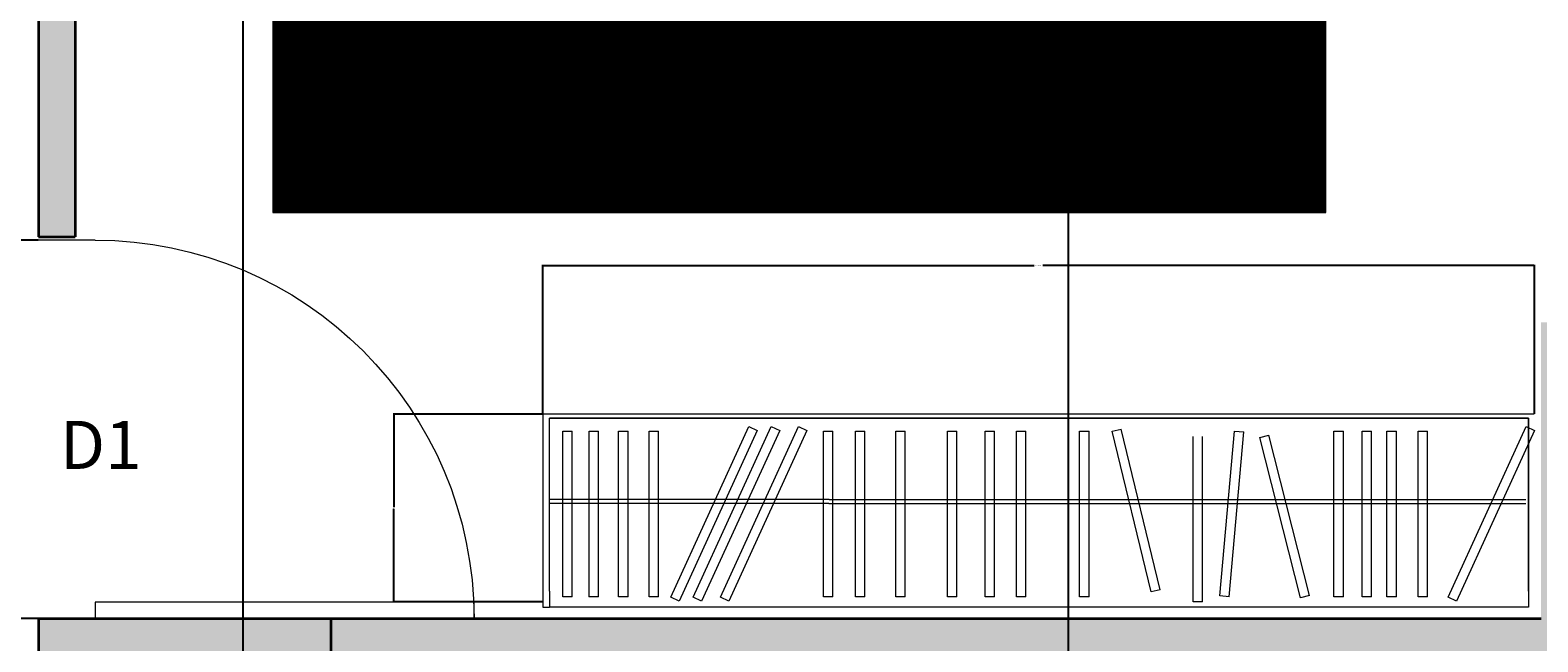
# Model space of a CAD drawing. Units: inches. Extents: x 192 to 1361, y -1362 to 367.
# Tile 20 of 23: x 783 to 1153, y -454 to -304. Entities that reach past the tile are written whole.
import ezdxf

# ---------------------------------------------------------------- set-up
doc = ezdxf.new("R2010")
doc.units = ezdxf.units.IN
doc.header["$MEASUREMENT"] = 0
for name, color, linetype, lineweight in [('A-ANNO-DIMS', 2, 'Continuous', 18), ('A-DOOR', 4, 'Continuous', 18), ('A-FLOR', 8, 'Continuous', 18), ('A-WALL-PATT', 250, 'Continuous', 13), ('closet', 32, 'Continuous', 18), ('text', 7, 'Continuous', 18), ('walls', 7, 'Continuous', 35)]:
    doc.layers.add(name, color=color, linetype=linetype, lineweight=lineweight)
doc.layers.add('A-FLOR-PATT', color=254, linetype='Continuous', lineweight=13, true_color=0xfeeab9)
doc.styles.get("Standard").update_dxf_attribs({"font": 'arial.ttf'})
doc.dimstyles.get("Standard").update_dxf_attribs({"dimtxt": 0.18, "dimasz": 0.18, "dimexe": 0.18, "dimexo": 0.0625, "dimgap": 0.09, "dimtad": 0, "dimtih": 1, "dimtoh": 1, "dimzin": 0, "dimdsep": 46, "dimlunit": 3, "dimtxsty": 'Standard', "dimcen": 0.09, "dimadec": 0, "dimazin": 0, "dimtfac": 1, "dimtofl": 0, "dimtmove": 0, "dimatfit": 3, "dimfxl": 1, "dimtolj": 1, "dimtzin": 0, "dimarcsym": 0})

# ---------------------------------------------------------------- blocks, each defined once
blk = doc.blocks.new('*U2')
for p, q in [((0, 0), (0, -6)), ((40, 0), (40, -6))]:
    blk.add_line(p, q)
blk.add_lwpolyline([(0, 0), (0, 40), (1.75, 40), (1.75, 0)], close=True)
blk.add_arc((0, 0), 40, 0, 90)
blk = doc.blocks.new('closet')
at = {"layer": 'closet'}
for p, q in [((-0.71, -5.58), (5.59, 8.19)), ((-0.23, 7.39), (-0.23, -6.57)), ((6.27, 7.88), (-0.04, -5.89)), ((5.59, 8.19), (6.27, 7.88)), ((7.92, 7.84), (8.68, 7.84)), ((7.92, 7.84), (7.92, -5.51)), ((8.68, 7.84), (8.68, -5.51)), ((10.44, 7.84), (11.2, 7.84)), ((10.44, 7.84), (10.44, -5.51)), ((11.2, 7.84), (11.2, -5.51)), ((12.45, 7.84), (13.21, 7.84)), ((12.45, 7.84), (12.45, -5.51)), ((13.21, 7.84), (13.21, -5.51)), ((14.71, 7.84), (15.47, 7.84)), ((14.71, 7.84), (14.71, -5.51)), ((15.47, 7.84), (15.47, -5.51)), ((17.44, 7.75), (18.17, 7.93)), ((17.44, 7.75), (20.73, -5.2)), ((18.17, 7.93), (21.46, -5.01)), ((23.92, 7.84), (22.75, -5.46)), ((24.67, 7.78), (23.51, -5.53)), ((23.92, 7.84), (24.67, 7.78)), ((26.09, 8.25), (26.09, -5.1)), ((26.84, 8.25), (26.84, -5.1)), ((30.22, 7.46), (33.37, -5.51)), ((35.23, 7.84), (35.23, -5.51)), ((35.99, 7.84), (35.99, -5.51)), ((40.33, 7.84), (40.33, -5.51)), ((41.08, 7.84), (41.08, -5.51)), ((42.85, 7.84), (42.85, -5.51)), ((43.61, 7.84), (43.61, -5.51)), ((45.9, 7.84), (45.9, -5.51)), ((46.65, 7.84), (46.65, -5.51)), ((50.07, 7.84), (50.07, -5.51)), ((50.82, 7.84), (50.82, -5.51)), ((53.32, 7.84), (53.32, -5.51)), ((54.08, 7.84), (54.08, -5.51)), ((55.9, 7.84), (55.9, -5.51)), ((56.65, 7.84), (56.65, -5.51)), ((57.99, -5.58), (64.3, 8.19)), ((64.97, 7.88), (58.67, -5.89)), ((60.19, -5.58), (66.49, 8.19)), ((67.17, 7.88), (60.87, -5.89)), ((62, -5.58), (68.3, 8.19)), ((68.98, 7.88), (62.67, -5.89)), ((69.96, 7.84), (69.96, -5.51)), ((70.72, 7.84), (70.72, -5.51)), ((72.43, 7.84), (72.43, -5.51)), ((73.19, 7.84), (73.19, -5.51)), ((74.82, 7.84), (74.82, -5.51)), ((75.57, 7.84), (75.57, -5.51)), ((76.94, 7.84), (76.94, -5.51)), ((77.69, 7.84), (77.69, -5.51)), ((29.49, 7.29), (32.64, -5.69)), ((56.23, 0.33), (0, 0.33)), ((56.2, 0), (0, 0)), ((56.2, 0), (78.76, 0)), ((56.23, 0.33), (78.76, 0.33)), ((-0.04, -5.89), (-0.71, -5.58)), ((21.46, -5.01), (20.73, -5.2)), ((23.51, -5.53), (22.75, -5.46)), ((33.37, -5.51), (32.64, -5.69)), ((35.99, -5.51), (35.23, -5.51)), ((41.08, -5.51), (40.33, -5.51)), ((43.61, -5.51), (42.85, -5.51)), ((46.65, -5.51), (45.9, -5.51)), ((50.82, -5.51), (50.07, -5.51)), ((54.08, -5.51), (53.32, -5.51)), ((56.65, -5.51), (55.9, -5.51)), ((58.67, -5.89), (57.99, -5.58)), ((60.87, -5.89), (60.19, -5.58)), ((62.67, -5.89), (62, -5.58)), ((70.72, -5.51), (69.96, -5.51)), ((73.19, -5.51), (72.43, -5.51)), ((75.57, -5.51), (74.82, -5.51)), ((77.69, -5.51), (76.94, -5.51))]:
    blk.add_line(p, q, dxfattribs=at)
blk = doc.blocks.new('rotated closet')
at = {"layer": 'closet'}
for p, q in [((26.32, 0.86), (27.07, 0.86)), ((29.72, -0.11), (30.45, 0.07)), ((35.46, 0.45), (36.22, 0.45)), ((40.56, 0.45), (41.31, 0.45)), ((43.08, 0.45), (43.84, 0.45)), ((46.13, 0.45), (46.88, 0.45)), ((50.3, 0.45), (51.05, 0.45)), ((53.56, 0.45), (54.31, 0.45)), ((56.13, 0.45), (56.88, 0.45)), ((64.53, 0.8), (65.2, 0.49)), ((66.72, 0.8), (67.4, 0.49)), ((68.53, 0.8), (69.21, 0.49)), ((70.19, 0.45), (70.95, 0.45)), ((72.66, 0.45), (73.42, 0.45)), ((75.05, 0.45), (75.81, 0.45)), ((77.17, 0.45), (77.92, 0.45)), ((78.99, 0), (78.99, -13.96)), ((8.91, -12.91), (8.15, -12.91)), ((11.43, -12.91), (10.67, -12.91)), ((13.44, -12.91), (12.68, -12.91)), ((15.7, -12.91), (14.94, -12.91)), ((-0.46, -14.27), (79.54, -14.27)), ((0, -13.96), (78.99, -13.96))]:
    blk.add_line(p, q, dxfattribs=at)
blk.add_blockref('closet', (0.23, -7.39), dxfattribs=at)
blk = doc.blocks.new('*D29')
at = {"layer": 'A-ANNO-DIMS', "color": 0, "lineweight": -2, "transparency": 16777216}
for p, q in [((908.62, -398.22), (908.62, -361.57)), ((908.8, -361.75), (1029.33, -361.75)), ((1152, -361.75), (1031.47, -361.75)), ((1152.18, -398.22), (1152.18, -361.57))]:
    blk.add_line(p, q, dxfattribs=at)
at = {"layer": 'A-ANNO-DIMS', "color": 0, "transparency": 16777216}
for points in [[(908.8, -361.72), (908.8, -361.78), (908.62, -361.75)], [(1152, -361.72), (1152, -361.78), (1152.18, -361.75)]]:
    blk.add_solid(points, dxfattribs=at)
at = {"layer": 'Defpoints', "color": 0, "transparency": 16777216}
for p in [(908.62, -361.75), (908.62, -398.29), (1152.18, -398.29)]:
    blk.add_point(p, dxfattribs=at)
at = {"layer": 'A-ANNO-DIMS', "color": 0, "transparency": 16777216, "insert": (1030.4, -361.75), "char_height": 0.18, "attachment_point": 5}
blk.add_mtext('\\A1;WARDROBE 244', dxfattribs=at)
blk = doc.blocks.new('*D30')
at = {"layer": 'A-ANNO-DIMS', "color": 0, "lineweight": -2, "transparency": 16777216}
for p, q in [((908.56, -398.29), (871.91, -398.29)), ((872.09, -398.47), (872.09, -421.14)), ((872.09, -444.17), (872.09, -421.5)), ((908.56, -444.35), (871.91, -444.35))]:
    blk.add_line(p, q, dxfattribs=at)
at = {"layer": 'A-ANNO-DIMS', "color": 0, "transparency": 16777216}
for points in [[(872.06, -398.47), (872.12, -398.47), (872.09, -398.29)], [(872.06, -444.17), (872.12, -444.17), (872.09, -444.35)]]:
    blk.add_solid(points, dxfattribs=at)
at = {"layer": 'Defpoints', "color": 0, "transparency": 16777216}
for p in [(908.62, -398.29), (872.09, -444.35), (908.62, -444.35)]:
    blk.add_point(p, dxfattribs=at)
at = {"layer": 'A-ANNO-DIMS', "color": 0, "transparency": 16777216, "insert": (872.09, -421.32), "char_height": 0.18, "attachment_point": 5}
blk.add_mtext('\\A1;46', dxfattribs=at)
blk = doc.blocks.new('*D71')
at = {"layer": 'A-ANNO-DIMS', "color": 0, "lineweight": -2, "transparency": 16777216}
for p, q in [((784.74, -355.5), (192.16, -355.5)), ((192.34, -355.68), (192.34, -401.82)), ((192.34, -448.32), (192.34, -402.18)), ((784.74, -448.5), (192.16, -448.5))]:
    blk.add_line(p, q, dxfattribs=at)
at = {"layer": 'A-ANNO-DIMS', "color": 0, "transparency": 16777216}
for points in [[(192.31, -355.68), (192.37, -355.68), (192.34, -355.5)], [(192.31, -448.32), (192.37, -448.32), (192.34, -448.5)]]:
    blk.add_solid(points, dxfattribs=at)
at = {"layer": 'Defpoints', "color": 0, "transparency": 16777216}
for p in [(784.8, -355.5), (192.34, -448.5), (784.8, -448.5)]:
    blk.add_point(p, dxfattribs=at)
at = {"layer": 'A-ANNO-DIMS', "color": 0, "transparency": 16777216, "insert": (192.34, -402), "char_height": 0.18, "attachment_point": 5}
blk.add_mtext('\\A1;93', dxfattribs=at)
blk = doc.blocks.new('*D72')
at = {"layer": 'A-ANNO-DIMS', "color": 0, "lineweight": -2, "transparency": 16777216}
for p, q in [((835.08, -1067.56), (835.08, 367.39)), ((835.26, 367.21), (935.95, 367.21)), ((1037.58, 367.21), (936.88, 367.21)), ((1037.76, -1067.56), (1037.76, 367.39))]:
    blk.add_line(p, q, dxfattribs=at)
at = {"layer": 'A-ANNO-DIMS', "color": 0, "transparency": 16777216}
for points in [[(835.26, 367.24), (835.26, 367.18), (835.08, 367.21)], [(1037.58, 367.24), (1037.58, 367.18), (1037.76, 367.21)]]:
    blk.add_solid(points, dxfattribs=at)
at = {"layer": 'Defpoints', "color": 0, "transparency": 16777216}
for p in [(1037.76, 367.21), (835.08, -1067.62), (1037.76, -1067.62)]:
    blk.add_point(p, dxfattribs=at)
at = {"layer": 'A-ANNO-DIMS', "color": 0, "transparency": 16777216, "insert": (936.42, 367.21), "char_height": 0.18, "attachment_point": 5}
blk.add_mtext('\\A1;202.68', dxfattribs=at)

msp = doc.modelspace()

# ---------------------------------------------------------------- hatches: boundary and pattern name
at = {"layer": 'A-FLOR-PATT'}
h = msp.add_hatch(dxfattribs=at)
h.set_pattern_fill('ANSI31', color=256)
edge = h.paths.add_edge_path()
edge.add_line((1100.9659, -111.2666), (1078.5607, -111.2666))
edge.add_line((1078.5607, -111.2666), (1045.5537, -110.9483))
edge.add_line((1045.5537, -110.9483), (1045.5537, -185.8956))
edge.add_line((1045.5537, -185.8956), (1065.0331, -185.8956))
edge.add_line((1065.0331, -185.8956), (1065.0331, -267.8066))
edge.add_line((1065.0331, -267.8066), (868.5929, -267.8066))
edge.add_line((868.5929, -267.8066), (868.5929, -267.2863))
edge.add_spline(control_points=[(865.1222, -267.5809), (865.4243, -267.2044), (866.0209, -266.461), (867.0867, -267.2043), (867.9397, -267.7344), (868.3935, -267.4276), (868.5929, -267.2863)], knot_values=[0, 0, 0, 0, 0.65327829, 1.2901376, 1.74045698, 2.09412198, 2.09412198, 2.09412198, 2.09412198], degree=3, periodic=0)
edge.add_line((868.5929, -267.2863), (868.5929, -265.8146))
edge.add_spline(control_points=[(865.1222, -266.1092), (865.4243, -265.7327), (866.0209, -264.9893), (867.0867, -265.7326), (867.9397, -266.2626), (868.3935, -265.9559), (868.5929, -265.8146)], knot_values=[0, 0, 0, 0, 0.65327829, 1.2901376, 1.74045698, 2.09412198, 2.09412198, 2.09412198, 2.09412198], degree=3, periodic=0)
edge.add_line((868.5929, -265.8146), (868.5929, -264.3081))
edge.add_spline(control_points=[(865.1222, -264.6026), (865.4243, -264.2262), (866.0209, -263.4827), (867.0867, -264.2261), (867.9397, -264.7561), (868.3935, -264.4493), (868.5929, -264.3081)], knot_values=[0, 0, 0, 0, 0.65327829, 1.2901376, 1.74045698, 2.09412198, 2.09412198, 2.09412198, 2.09412198], degree=3, periodic=0)
edge.add_line((868.5929, -264.3081), (868.5929, -263.0738))
edge.add_spline(control_points=[(865.1222, -263.3684), (865.4243, -262.9919), (866.0209, -262.2485), (867.0867, -262.9918), (867.9397, -263.5219), (868.3935, -263.2151), (868.5929, -263.0738)], knot_values=[0, 0, 0, 0, 0.65327829, 1.2901376, 1.74045698, 2.09412198, 2.09412198, 2.09412198, 2.09412198], degree=3, periodic=0)
edge.add_line((868.5929, -263.0738), (868.5929, -259.0322))
edge.add_spline(control_points=[(865.1222, -259.3268), (865.4242, -258.9505), (866.0208, -258.2073), (867.0871, -258.949), (867.938, -259.4827), (868.3932, -259.1696), (868.5929, -259.0322)], knot_values=[0, 0, 0, 0, 0.65327829, 1.2901376, 1.74045698, 2.09260048, 2.09260048, 2.09260048, 2.09260048], degree=3, periodic=0)
edge.add_line((868.5929, -259.0322), (868.5929, -255.8497))
edge.add_spline(control_points=[(865.1222, -256.1443), (865.4242, -255.768), (866.0208, -255.0247), (867.0871, -255.7664), (867.938, -256.3002), (868.3932, -255.9871), (868.5929, -255.8497)], knot_values=[0, 0, 0, 0, 0.65327829, 1.2901376, 1.74045698, 2.09260048, 2.09260048, 2.09260048, 2.09260048], degree=3, periodic=0)
edge.add_line((868.5929, -255.8497), (868.5929, -253.1089))
edge.add_spline(control_points=[(865.1222, -253.4035), (865.4242, -253.0272), (866.0208, -252.284), (867.0871, -253.0257), (867.938, -253.5594), (868.3932, -253.2463), (868.5929, -253.1089)], knot_values=[0, 0, 0, 0, 0.65327829, 1.2901376, 1.74045698, 2.09260048, 2.09260048, 2.09260048, 2.09260048], degree=3, periodic=0)
edge.add_line((868.5929, -253.1089), (868.5929, -250.8478))
edge.add_spline(control_points=[(865.1222, -251.1424), (865.4243, -250.766), (866.0209, -250.0225), (867.0867, -250.7659), (867.9397, -251.2959), (868.3935, -250.9891), (868.5929, -250.8478)], knot_values=[0, 0, 0, 0, 0.65327829, 1.2901376, 1.74045698, 2.09412198, 2.09412198, 2.09412198, 2.09412198], degree=3, periodic=0)
edge.add_line((868.5929, -250.8478), (868.5929, -248.511))
edge.add_spline(control_points=[(865.1222, -248.8056), (865.4243, -248.4291), (866.0209, -247.6857), (867.0867, -248.429), (867.9397, -248.9591), (868.3935, -248.6523), (868.5929, -248.511)], knot_values=[0, 0, 0, 0, 0.65327829, 1.2901376, 1.74045698, 2.09412198, 2.09412198, 2.09412198, 2.09412198], degree=3, periodic=0)
edge.add_line((868.5929, -248.511), (868.5929, -245.7702))
edge.add_spline(control_points=[(865.1222, -246.0648), (865.4243, -245.6884), (866.0209, -244.9449), (867.0867, -245.6883), (867.9397, -246.2183), (868.3935, -245.9115), (868.5929, -245.7702)], knot_values=[0, 0, 0, 0, 0.65327829, 1.2901376, 1.74045698, 2.09412198, 2.09412198, 2.09412198, 2.09412198], degree=3, periodic=0)
edge.add_line((868.5929, -245.7702), (868.5929, -243.5091))
edge.add_spline(control_points=[(865.1222, -243.8037), (865.4243, -243.4273), (866.0209, -242.6838), (867.0867, -243.4272), (867.9397, -243.9572), (868.3935, -243.6504), (868.5929, -243.5091)], knot_values=[0, 0, 0, 0, 0.65327829, 1.2901376, 1.74045698, 2.09412198, 2.09412198, 2.09412198, 2.09412198], degree=3, periodic=0)
edge.add_line((868.5929, -243.5091), (868.5929, -240.974))
edge.add_spline(control_points=[(865.1222, -241.2686), (865.4243, -240.8921), (866.0209, -240.1487), (867.0867, -240.892), (867.9397, -241.422), (868.3935, -241.1153), (868.5929, -240.974)], knot_values=[0, 0, 0, 0, 0.65327829, 1.2901376, 1.74045698, 2.09412198, 2.09412198, 2.09412198, 2.09412198], degree=3, periodic=0)
edge.add_line((868.5929, -240.974), (868.5929, -238.832))
edge.add_spline(control_points=[(865.1222, -239.1266), (865.4243, -238.7501), (866.0209, -238.0067), (867.0867, -238.75), (867.9397, -239.2801), (868.3935, -238.9733), (868.5929, -238.832)], knot_values=[0, 0, 0, 0, 0.65327829, 1.2901376, 1.74045698, 2.09412198, 2.09412198, 2.09412198, 2.09412198], degree=3, periodic=0)
edge.add_line((868.5929, -238.832), (868.5929, -236.2969))
edge.add_spline(control_points=[(865.1222, -236.5915), (865.4243, -236.215), (866.0209, -235.4715), (867.0867, -236.2149), (867.9397, -236.7449), (868.3935, -236.4382), (868.5929, -236.2969)], knot_values=[0, 0, 0, 0, 0.65327829, 1.2901376, 1.74045698, 2.09412198, 2.09412198, 2.09412198, 2.09412198], degree=3, periodic=0)
edge.add_line((868.5929, -236.2969), (868.5929, -233.5562))
edge.add_spline(control_points=[(865.1222, -233.8508), (865.4243, -233.4743), (866.0209, -232.7309), (867.0867, -233.4742), (867.9397, -234.0042), (868.3935, -233.6975), (868.5929, -233.5562)], knot_values=[0, 0, 0, 0, 0.65327829, 1.2901376, 1.74045698, 2.09412198, 2.09412198, 2.09412198, 2.09412198], degree=3, periodic=0)
edge.add_line((868.5929, -233.5562), (868.5929, -230.3358))
edge.add_spline(control_points=[(865.1222, -230.6304), (865.4243, -230.254), (866.0209, -229.5105), (867.0867, -230.2539), (867.9397, -230.7839), (868.3935, -230.4771), (868.5929, -230.3358)], knot_values=[0, 0, 0, 0, 0.65327829, 1.2901376, 1.74045698, 2.09412198, 2.09412198, 2.09412198, 2.09412198], degree=3, periodic=0)
edge.add_line((868.5929, -230.3358), (868.5929, -227.5951))
edge.add_spline(control_points=[(865.1222, -227.8896), (865.4243, -227.5132), (866.0209, -226.7697), (867.0867, -227.5131), (867.9397, -228.0431), (868.3935, -227.7363), (868.5929, -227.5951)], knot_values=[0, 0, 0, 0, 0.65327829, 1.2901376, 1.74045698, 2.09412198, 2.09412198, 2.09412198, 2.09412198], degree=3, periodic=0)
edge.add_line((868.5929, -227.5951), (868.5929, -225.334))
edge.add_spline(control_points=[(865.1222, -225.6285), (865.4243, -225.2521), (866.0209, -224.5086), (867.0867, -225.252), (867.9397, -225.782), (868.3935, -225.4752), (868.5929, -225.334)], knot_values=[0, 0, 0, 0, 0.65327829, 1.2901376, 1.74045698, 2.09412198, 2.09412198, 2.09412198, 2.09412198], degree=3, periodic=0)
edge.add_line((868.5929, -225.334), (868.5929, -222.9971))
edge.add_spline(control_points=[(865.1222, -223.2917), (865.4243, -222.9153), (866.0209, -222.1718), (867.0867, -222.9152), (867.9397, -223.4452), (868.3935, -223.1384), (868.5929, -222.9971)], knot_values=[0, 0, 0, 0, 0.65327829, 1.2901376, 1.74045698, 2.09412198, 2.09412198, 2.09412198, 2.09412198], degree=3, periodic=0)
edge.add_line((868.5929, -222.9971), (868.5929, -220.2564))
edge.add_spline(control_points=[(865.1222, -220.5509), (865.4243, -220.1745), (866.0209, -219.431), (867.0867, -220.1744), (867.9397, -220.7044), (868.3935, -220.3976), (868.5929, -220.2564)], knot_values=[0, 0, 0, 0, 0.65327829, 1.2901376, 1.74045698, 2.09412198, 2.09412198, 2.09412198, 2.09412198], degree=3, periodic=0)
edge.add_line((868.5929, -220.2564), (868.5929, -217.9953))
edge.add_spline(control_points=[(865.1222, -218.2898), (865.4243, -217.9134), (866.0209, -217.1699), (867.0867, -217.9133), (867.9397, -218.4433), (868.3935, -218.1365), (868.5929, -217.9953)], knot_values=[0, 0, 0, 0, 0.65327829, 1.2901376, 1.74045698, 2.09412198, 2.09412198, 2.09412198, 2.09412198], degree=3, periodic=0)
edge.add_line((868.5929, -217.9953), (868.5929, -215.4601))
edge.add_spline(control_points=[(865.1222, -215.7547), (865.4243, -215.3782), (866.0209, -214.6348), (867.0867, -215.3781), (867.9397, -215.9082), (868.3935, -215.6014), (868.5929, -215.4601)], knot_values=[0, 0, 0, 0, 0.65327829, 1.2901376, 1.74045698, 2.09412198, 2.09412198, 2.09412198, 2.09412198], degree=3, periodic=0)
edge.add_line((868.5929, -215.4601), (868.5929, -213.0475))
edge.add_spline(control_points=[(865.1222, -213.3421), (865.4243, -212.9656), (866.0209, -212.2222), (867.0867, -212.9655), (867.9397, -213.4955), (868.3935, -213.1888), (868.5929, -213.0475)], knot_values=[0, 0, 0, 0, 0.65327829, 1.2901376, 1.74045698, 2.09412198, 2.09412198, 2.09412198, 2.09412198], degree=3, periodic=0)
edge.add_line((868.5929, -213.0475), (868.5929, -210.5123))
edge.add_spline(control_points=[(865.1222, -210.8069), (865.4243, -210.4305), (866.0209, -209.687), (867.0867, -210.4304), (867.9397, -210.9604), (868.3935, -210.6536), (868.5929, -210.5123)], knot_values=[0, 0, 0, 0, 0.65327829, 1.2901376, 1.74045698, 2.09412198, 2.09412198, 2.09412198, 2.09412198], degree=3, periodic=0)
edge.add_line((868.5929, -210.5123), (868.5929, -207.7717))
edge.add_spline(control_points=[(865.1222, -208.0662), (865.4243, -207.6898), (866.0209, -206.9463), (867.0867, -207.6897), (867.9397, -208.2197), (868.3935, -207.9129), (868.5929, -207.7717)], knot_values=[0, 0, 0, 0, 0.65327829, 1.2901376, 1.74045698, 2.09412198, 2.09412198, 2.09412198, 2.09412198], degree=3, periodic=0)
edge.add_line((868.5929, -207.7717), (868.5929, -204.5513))
edge.add_spline(control_points=[(865.1222, -204.8459), (865.4243, -204.4694), (866.0209, -203.726), (867.0867, -204.4693), (867.9397, -204.9993), (868.3935, -204.6926), (868.5929, -204.5513)], knot_values=[0, 0, 0, 0, 0.65327829, 1.2901376, 1.74045698, 2.09412198, 2.09412198, 2.09412198, 2.09412198], degree=3, periodic=0)
edge.add_line((868.5929, -204.5513), (868.5929, -201.8105))
edge.add_spline(control_points=[(865.1222, -202.1051), (865.4243, -201.7286), (866.0209, -200.9852), (867.0867, -201.7285), (867.9397, -202.2586), (868.3935, -201.9518), (868.5929, -201.8105)], knot_values=[0, 0, 0, 0, 0.65327829, 1.2901376, 1.74045698, 2.09412198, 2.09412198, 2.09412198, 2.09412198], degree=3, periodic=0)
edge.add_line((868.5929, -201.8105), (868.5929, -199.5494))
edge.add_spline(control_points=[(865.1222, -199.844), (865.4243, -199.4675), (866.0209, -198.7241), (867.0867, -199.4674), (867.9397, -199.9975), (868.3935, -199.6907), (868.5929, -199.5494)], knot_values=[0, 0, 0, 0, 0.65327829, 1.2901376, 1.74045698, 2.09412198, 2.09412198, 2.09412198, 2.09412198], degree=3, periodic=0)
edge.add_line((868.5929, -199.5494), (868.5929, -197.2126))
edge.add_spline(control_points=[(865.1222, -197.5072), (865.4243, -197.1307), (866.0209, -196.3873), (867.0867, -197.1306), (867.9397, -197.6606), (868.3935, -197.3539), (868.5929, -197.2126)], knot_values=[0, 0, 0, 0, 0.65327829, 1.2901376, 1.74045698, 2.09412198, 2.09412198, 2.09412198, 2.09412198], degree=3, periodic=0)
edge.add_line((868.5929, -197.2126), (868.5929, -194.4718))
edge.add_spline(control_points=[(865.1222, -194.7664), (865.4243, -194.3899), (866.0209, -193.6465), (867.0867, -194.3898), (867.9397, -194.9199), (868.3935, -194.6131), (868.5929, -194.4718)], knot_values=[0, 0, 0, 0, 0.65327829, 1.2901376, 1.74045698, 2.09412198, 2.09412198, 2.09412198, 2.09412198], degree=3, periodic=0)
edge.add_line((868.5929, -194.4718), (868.5929, -192.2107))
edge.add_spline(control_points=[(865.1222, -192.5053), (865.4243, -192.1288), (866.0209, -191.3854), (867.0867, -192.1288), (867.9397, -192.6588), (868.3935, -192.352), (868.5929, -192.2107)], knot_values=[0, 0, 0, 0, 0.65327829, 1.2901376, 1.74045698, 2.09412198, 2.09412198, 2.09412198, 2.09412198], degree=3, periodic=0)
edge.add_line((868.5929, -192.2107), (868.5929, -189.6756))
edge.add_spline(control_points=[(865.1222, -189.9702), (865.4243, -189.5937), (866.0209, -188.8502), (867.0867, -189.5936), (867.9397, -190.1236), (868.3935, -189.8169), (868.5929, -189.6756)], knot_values=[0, 0, 0, 0, 0.65327829, 1.2901376, 1.74045698, 2.09412198, 2.09412198, 2.09412198, 2.09412198], degree=3, periodic=0)
edge.add_line((868.5929, -189.6756), (868.5929, -187.259))
edge.add_spline(control_points=[(865.1222, -187.5536), (865.4243, -187.1771), (866.0209, -186.4337), (867.0867, -187.177), (867.9397, -187.7071), (868.3935, -187.4003), (868.5929, -187.259)], knot_values=[0, 0, 0, 0, 0.65327829, 1.2901376, 1.74045698, 2.09412198, 2.09412198, 2.09412198, 2.09412198], degree=3, periodic=0)
edge.add_line((868.5929, -187.259), (868.5929, -185.8956))
edge.add_line((868.5929, -185.8956), (898.2296, -185.8956))
edge.add_line((898.2296, -185.8956), (898.2296, -110.9483))
edge.add_line((898.2296, -110.9483), (865.2226, -110.63))
edge.add_line((865.2226, -110.63), (842.3259, -110.63))
edge.add_line((842.3259, -110.63), (842.3259, -348.7284))
edge.add_line((842.3259, -348.7284), (1100.9659, -348.7284))
edge.add_line((1100.9659, -348.7284), (1100.9659, -111.2666))
at = {"layer": 'A-WALL-PATT'}
h = msp.add_hatch(color=256, dxfattribs=at)
h.dxf.hatch_style = 1
h.paths.add_polyline_path([(309.5452, 191.102), (300.5452, 191.102), (300.5452, -126.898), (309.5452, -126.898), (309.5452, -117.898)])
h.paths.add_polyline_path([(420.798, 191.102), (337.3229, 191.102), (337.3229, 182.102), (420.798, 182.102)])
h.paths.add_polyline_path([(518.5452, 182.102), (625.4022, 182.102), (625.4022, 191.102), (509.5452, 191.102), (509.5452, 114.3262), (518.5452, 114.3262)])
h.paths.add_polyline_path([(842.5452, 191.102), (763.4438, 191.102), (763.4438, 182.102), (833.5452, 182.102), (833.5452, 161.1615), (836.8088, 161.1615), (842.5452, 161.1615)])
h.paths.add_polyline_path([(842.5452, -16.5675), (833.5452, -16.5675), (833.5452, -60.4996), (784.8041, -60.4996), (784.8041, -354.6796), (793.8041, -354.6796), (793.8041, -69.4996), (1094.1252, -69.4996), (1094.1252, -60.4996), (842.5452, -60.4996)])
h.paths.add_polyline_path([(518.5452, 36.602), (509.5452, 36.602), (509.5452, -117.898), (420.2204, -117.898), (420.2204, -126.898), (518.5452, -126.898)])
h.paths.add_polyline_path([(474.8041, -377.0384), (465.8041, -377.0384), (465.8041, -381.5384), (465.8041, -450.898), (537.5717, -450.898), (537.5717, -441.898), (474.8041, -441.898)])
h.paths.add_polyline_path([(1162.8041, -380.6763), (1204.3001, -380.6763), (1204.3001, -375.6763), (1195.1471, -375.6763), (1153.8041, -375.6763), (1153.8041, -448.4996), (856.5691, -448.4996), (856.5691, -457.4996), (1162.8041, -457.4996)])
h.paths.add_polyline_path([(1162.8041, -525.128), (1153.8041, -525.128), (1153.8041, -597.4996), (1162.8041, -597.4996)], flags=17)
h.paths.add_polyline_path([(1162.8041, -60.4996), (1153.8041, -60.4996), (1153.8041, -69.4996), (1153.8041, -177.4733), (1205.8889, -177.4733), (1205.8889, -172.4733), (1162.8041, -172.4733)])
h.paths.add_polyline_path([(980.5799, -525.686), (971.5799, -525.686), (971.5799, -597.4996), (980.5799, -597.4996)], flags=17)
h.paths.add_polyline_path([(856.5691, -448.4996), (798.7542, -448.4996), (784.8041, -448.4996), (784.8041, -457.4996), (847.5691, -457.4996), (847.5691, -597.4996), (784.8041, -597.4996), (784.8041, -606.4996), (1273.5658, -606.4996), (1273.5658, -597.4996), (856.5691, -597.4996)])
h.paths.add_polyline_path([(1273.5658, -773.892), (1099.8366, -773.892), (1099.8366, -851.9362), (1108.8366, -851.9362), (1108.8366, -782.892), (1273.5658, -782.892)])
h.paths.add_polyline_path([(1108.8366, -982.9214), (1099.8366, -982.9214), (1099.8366, -1067.6246), (1037.7563, -1067.6246), (1037.7563, -1076.6246), (1108.8366, -1076.6246)])
h.paths.add_polyline_path([(835.078, -1067.6246), (758.8458, -1067.6246), (758.8458, -940.2324), (749.8458, -940.2324), (749.8458, -963.172), (749.8458, -970.4644), (749.8458, -1076.6246), (835.078, -1076.6246)])
h.paths.add_polyline_path([(450.307, -1066.9838), (441.307, -1066.9838), (441.307, -1076.6246), (450.307, -1076.6246)])
h.paths.add_polyline_path([(492.8925, -756.4415), (274.8925, -756.4415), (274.8925, -765.4415), (492.8925, -765.4415)])
h.paths.add_polyline_path([(283.8925, -835.2244), (274.8925, -835.2244), (274.8925, -914.4415), (492.8925, -914.4415), (492.8925, -839.9415), (483.8925, -839.9415), (483.8925, -905.4415), (283.8925, -905.4415)])
h.paths.add_polyline_path([(283.8925, -441.898), (283.8925, -375.4296), (281.6021, -375.4296), (281.6021, -399.4121), (274.8925, -399.4121), (274.8925, -441.898), (274.8925, -684.5089), (283.8925, -684.5089)])

# ---------------------------------------------------------------- linework, layer by layer
at = {"layer": 'A-FLOR'}
for p, q in [((842.3259, -110.63), (842.3259, -348.7284)), ((1100.9659, -348.7284), (1100.9659, -111.2666)), ((842.3259, -348.7284), (1100.9659, -348.7284))]:
    msp.add_line(p, q, dxfattribs=at)
at = {"layer": 'closet'}
for p, q in [((1152.1073, -398.2873), (908.6207, -398.2873)), ((908.6207, -398.2873), (908.6207, -445.6684)), ((910.3094, -441.7326), (910.3094, -399.2454)), ((910.3094, -399.2454), (1150.7181, -399.2454)), ((1150.7181, -399.2454), (1150.7181, -441.7326)), ((910.3094, -441.7326), (910.3094, -445.6684)), ((1150.7181, -441.7326), (1150.7181, -445.6684)), ((908.6207, -445.6684), (910.3094, -445.6684)), ((1150.7181, -445.6684), (910.3094, -445.6684))]:
    msp.add_line(p, q, dxfattribs=at)
at = {"layer": 'walls'}
for p, q in [((784.8041, -60.4996), (784.8041, -354.6796)), ((793.8041, -69.4996), (793.8041, -354.6796)), ((784.8041, -354.6796), (793.8041, -354.6796)), ((784.8041, -448.4996), (1153.8041, -448.4996)), ((784.8041, -448.4996), (784.8041, -606.4996)), ((856.5691, -448.4996), (856.5691, -597.4996))]:
    msp.add_line(p, q, dxfattribs=at)

# ---------------------------------------------------------------- block references
at = {"layer": 'A-DOOR', "xscale": -2.325004183907831, "yscale": 2.325004183907831, "zscale": 2.325004183907831, "rotation": 270}
msp.add_blockref('*U2', (798.7542, -448.4996), dxfattribs=at)
at = {"layer": 'closet', "xscale": 3.043581746063057, "yscale": 3.043581746063057, "zscale": 3.043581746063057, "rotation": 179.9999999992007}
msp.add_blockref('rotated closet', (1150.7181, -441.7326), dxfattribs=at)

# ---------------------------------------------------------------- texts
at = {"layer": 'text'}
msp.add_text('D1', height=11.81288, dxfattribs=at).set_placement((790.0683, -411.7241))

# ---------------------------------------------------------------- dimensions: what is measured, and where the dimension line sits
at = {"layer": 'A-ANNO-DIMS'}
dim = msp.add_linear_dim(base=(1037.7563, 367.2097), p1=(835.078, -1067.6246), p2=(1037.7563, -1067.6246), dimstyle='Standard', override={"dimdec": 2, "dimlfac": 1, "dimrnd": 0, "dimzin": 0, "dimdsep": 46, "dimlunit": 2}, dxfattribs=at)
dim.commit()
dim.dimension.update_dxf_attribs({"geometry": '*D72', "text_midpoint": (936.4171, 367.2097)})
for base, p1, p2, angle, picture, middle in [((192.3425, -448.4996), (784.8041, -355.4994), (784.8041, -448.4996), 90, '*D71', (192.3425, -401.9995)), ((872.0869, -444.3494), (908.6207, -398.2873), (908.6207, -444.3494), 270, '*D30', (872.0869, -421.3184))]:
    dim = msp.add_linear_dim(base=base, p1=p1, p2=p2, angle=angle, dimstyle='Standard', override={"dimdec": 0, "dimlfac": 1, "dimrnd": 0, "dimzin": 0, "dimdsep": 46, "dimlunit": 2}, dxfattribs=at)
    dim.commit()
    dim.dimension.update_dxf_attribs({"geometry": picture, "text_midpoint": middle})
dim = msp.add_linear_dim(base=(908.6207, -361.7535), p1=(1152.1797, -398.2873), p2=(908.6207, -398.2873), angle=180, text='WARDROBE <>', dimstyle='Standard', override={"dimdec": 0, "dimlfac": 1, "dimrnd": 0, "dimzin": 0, "dimdsep": 46, "dimlunit": 2}, dxfattribs=at)
dim.commit()
dim.dimension.update_dxf_attribs({"geometry": '*D29', "text_midpoint": (1030.4002, -361.7535)})

doc.saveas('drawing.dxf')
